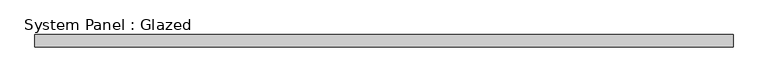
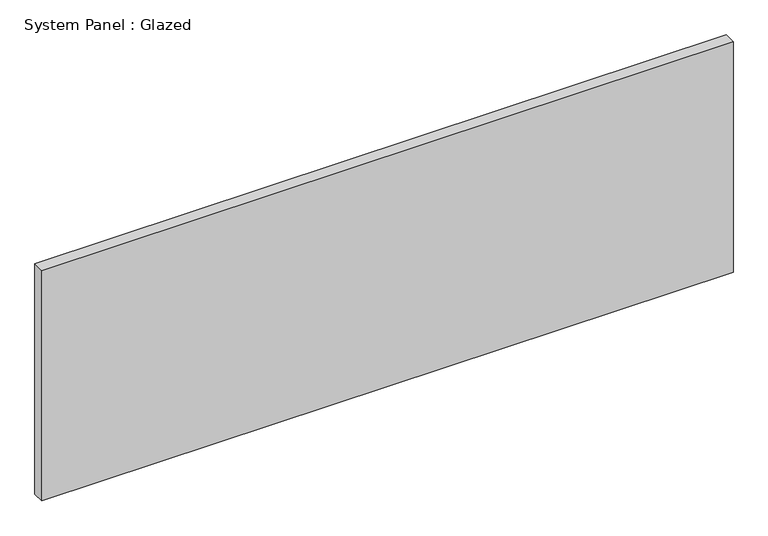
"""IFC4 building model written with IfcOpenShell, lengths in millimetres: plate geometry, System Panel : Glazed."""

from ifc_helpers import new_model, si_unit, origin, origin_with_axes, place, context, project, spatial, polyline, outline, extrude, source, transform, mapped, element, save


def system_panel_glazed_6dc8f8fc(model_context):
    return source(origin(), model_context, "Body", "SweptSolid", [
        extrude(outline(polyline([(730.2499999, 19.05), (-730.2499999, 19.05), (-730.2499999, 44.45), (730.2499999, 44.45), (730.2499999, 19.05)])), origin_with_axes(), (0.0, 0.0, 1.0), 514.35),
    ])


if __name__ == "__main__":
    model = new_model("IFC4")
    model_context = context("Model", 3, world=origin())
    ifc_project = project(units=[si_unit("LENGTHUNIT", "METRE", prefix="MILLI")], contexts=[model_context])
    site = spatial("IfcSite", under=ifc_project)
    building = spatial("IfcBuilding", under=site)
    placement = place(None, origin())
    system_panel_glazed_shape = system_panel_glazed_6dc8f8fc(model_context)
    element("IfcPlate", 1, ObjectType="System Panel : Glazed", at=placement, inside=building, context=model_context, shape_type="MappedRepresentation", body=[
        mapped(system_panel_glazed_shape, transform((0.0, 0.0, 0.0), x_axis=(1.0, 0.0, 0.0), y_axis=(0.0, 1.0, 0.0), z_axis=(0.0, 0.0, 1.0))),
    ])
    save(model, "model.ifc")

# Revit data of these elements
# Type "System Panel : Glazed"
#   Construction Type Id = "GSP4R"
#   Analytic Construction = "1/8 in Pilkington single glazing"
#   Visual Light Transmittance = 0.9
#   Solar Heat Gain Coefficient = 0.86
#   Heat Transfer Coefficient (U) = 1.18115 BTU/(h·ft²·°F)
#   Define Thermal Properties by = 1
# Element 1 (IfcPlate, "System Panel : Glazed")
#   Materials on its faces: "Glass"
# Materials
#   "Glass": class "Glass", colour RGB 0 128 192, transparency 0.75, Description = "Soda Lime Glass", Cost = 0
